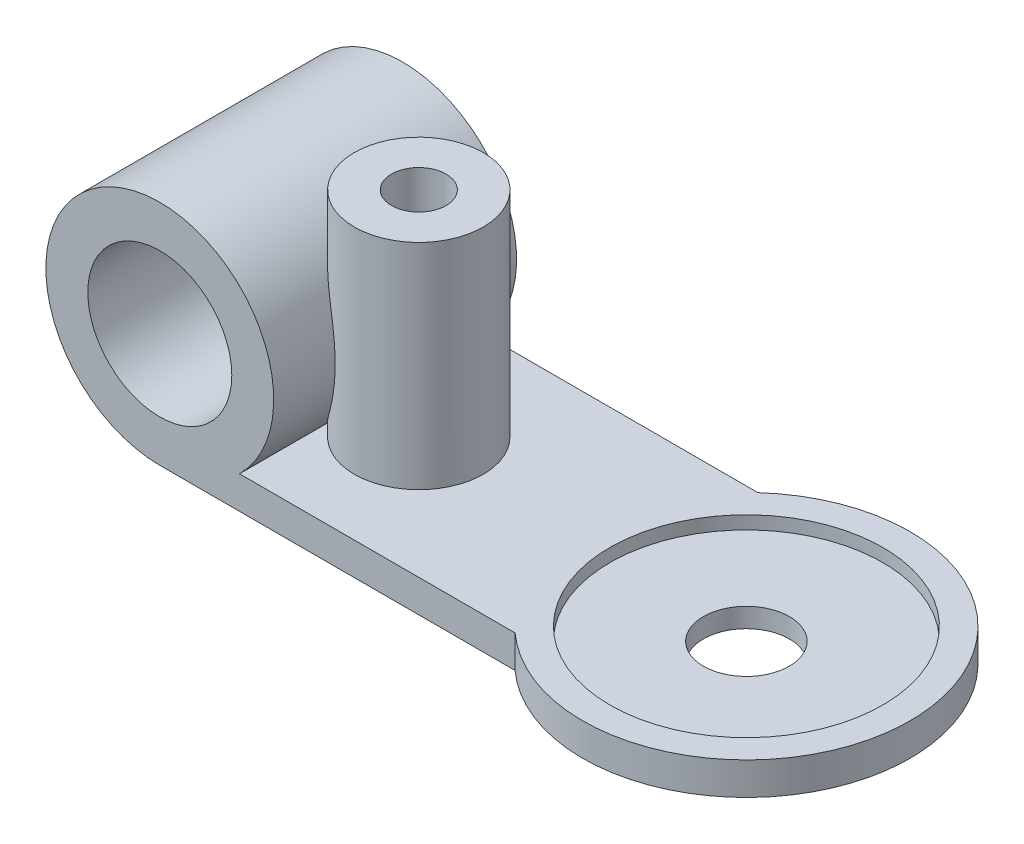
ISO-10303-21;
HEADER;
FILE_DESCRIPTION(('STEP AP214'),'2;1');
FILE_NAME('part.step','',(''),(''),'','','');
FILE_SCHEMA(('AUTOMOTIVE_DESIGN { 1 0 10303 214 1 1 1 1 }'));
ENDSEC;
DATA;
#1=APPLICATION_CONTEXT('core data for automotive mechanical design processes');
#2=APPLICATION_PROTOCOL_DEFINITION('international standard','automotive_design',2000,#1);
#3=PRODUCT_CONTEXT('',#1,'mechanical');
#4=PRODUCT('Part','Part','',(#3));
#5=PRODUCT_RELATED_PRODUCT_CATEGORY('part','',(#4));
#6=PRODUCT_DEFINITION_FORMATION('','',#4);
#7=PRODUCT_DEFINITION_CONTEXT('part definition',#1,'design');
#8=PRODUCT_DEFINITION('design','',#6,#7);
#9=PRODUCT_DEFINITION_SHAPE('','',#8);
#10=(LENGTH_UNIT() NAMED_UNIT(*) SI_UNIT(.MILLI.,.METRE.));
#11=(NAMED_UNIT(*) PLANE_ANGLE_UNIT() SI_UNIT($,.RADIAN.));
#12=(NAMED_UNIT(*) SI_UNIT($,.STERADIAN.) SOLID_ANGLE_UNIT());
#13=UNCERTAINTY_MEASURE_WITH_UNIT(LENGTH_MEASURE(1.E-05),#10,'distance_accuracy_value','');
#14=(GEOMETRIC_REPRESENTATION_CONTEXT(3) GLOBAL_UNCERTAINTY_ASSIGNED_CONTEXT((#13)) GLOBAL_UNIT_ASSIGNED_CONTEXT((#10,
#11,#12)) REPRESENTATION_CONTEXT('',''));
#15=CARTESIAN_POINT('',(0.,0.,0.));
#16=DIRECTION('',(0.,0.,1.));
#17=DIRECTION('',(1.,0.,0.));
#18=AXIS2_PLACEMENT_3D('',#15,#16,#17);
#19=CARTESIAN_POINT('',(0.,0.,28.25));
#20=DIRECTION('',(0.,0.,-1.));
#21=DIRECTION('',(-1.,0.,0.));
#22=AXIS2_PLACEMENT_3D('',#19,#20,#21);
#23=CYLINDRICAL_SURFACE('',#22,26.5);
#24=CARTESIAN_POINT('',(18.5395732151525,-18.935,-6.61943432400085));
#25=CARTESIAN_POINT('',(18.6184844088422,-18.857735922678,-6.7799048417251));
#26=CARTESIAN_POINT('',(18.6996500765237,-18.7772995053579,-6.93769789286287));
#27=CARTESIAN_POINT('',(18.8660127366865,-18.6101446090685,-7.24771071947177));
#28=CARTESIAN_POINT('',(18.9512093342821,-18.5234267450141,-7.39993103828863));
#29=CARTESIAN_POINT('',(19.2119367337667,-18.254144759126,-7.84758026850834));
#30=CARTESIAN_POINT('',(19.3928037608263,-18.0622597774062,-8.13439757428924));
#31=CARTESIAN_POINT('',(19.7627998857865,-17.6566247189803,-8.68095188456506));
#32=CARTESIAN_POINT('',(19.951837020215,-17.4430934524195,-8.94091496085011));
#33=CARTESIAN_POINT('',(20.3357805115592,-16.9939196843523,-9.43632416262915));
#34=CARTESIAN_POINT('',(20.5306880072531,-16.7582728736955,-9.67176549119735));
#35=CARTESIAN_POINT('',(20.9218465097154,-16.2672836439004,-10.1174184499874));
#36=CARTESIAN_POINT('',(21.1180906942836,-16.0120109229411,-10.3277131495032));
#37=CARTESIAN_POINT('',(21.5091176828609,-15.4827681042641,-10.7246923720679));
#38=CARTESIAN_POINT('',(21.7039005618658,-15.2087989734533,-10.9113781146592));
#39=CARTESIAN_POINT('',(22.0893971655171,-14.6432876309621,-11.2626874504629));
#40=CARTESIAN_POINT('',(22.2801010802677,-14.3517083671837,-11.4272619984179));
#41=CARTESIAN_POINT('',(22.654420937027,-13.7532508238555,-11.7353706091408));
#42=CARTESIAN_POINT('',(22.8380352807777,-13.4463691298775,-11.8788999476885));
#43=CARTESIAN_POINT('',(23.2748416317101,-12.6807752021044,-12.2055472513245));
#44=CARTESIAN_POINT('',(23.5230474379595,-12.2147374879152,-12.3782473299468));
#45=CARTESIAN_POINT('',(23.995092560242,-11.259213422958,-12.6886290410036));
#46=CARTESIAN_POINT('',(24.2189226548008,-10.7697182982629,-12.8262974468949));
#47=CARTESIAN_POINT('',(24.6387874594659,-9.77107435442968,-13.0717923879554));
#48=CARTESIAN_POINT('',(24.8347902467419,-9.26190380211747,-13.1795847828578));
#49=CARTESIAN_POINT('',(25.1961346386176,-8.22828073390988,-13.3697078714785));
#50=CARTESIAN_POINT('',(25.3614787423587,-7.70382946765761,-13.4520406409029));
#51=CARTESIAN_POINT('',(25.6629820174316,-6.63160021158971,-13.5967189298012));
#52=CARTESIAN_POINT('',(25.7984409213751,-6.08356320786244,-13.6585990242412));
#53=CARTESIAN_POINT('',(26.0343347911313,-4.97823420208279,-13.7632654845402));
#54=CARTESIAN_POINT('',(26.1347693571546,-4.42094209446301,-13.8060516324506));
#55=CARTESIAN_POINT('',(26.299813137327,-3.3001043780399,-13.8750090033395));
#56=CARTESIAN_POINT('',(26.364424374345,-2.73655912417212,-13.9011811644874));
#57=CARTESIAN_POINT('',(26.4573738854935,-1.60597799225613,-13.9384992548715));
#58=CARTESIAN_POINT('',(26.4857095319384,-1.03894186432941,-13.9496440955807));
#59=CARTESIAN_POINT('',(26.5078093563906,0.203223899776678,-13.958373278112));
#60=CARTESIAN_POINT('',(26.4940253741838,0.878523476463438,-13.9529958055844));
#61=CARTESIAN_POINT('',(26.4149873898834,2.22572657129171,-13.9215445875143));
#62=CARTESIAN_POINT('',(26.3497242849237,2.89762946766144,-13.8954671816726));
#63=CARTESIAN_POINT('',(26.1683420326795,4.23347916225571,-13.8203261304445));
#64=CARTESIAN_POINT('',(26.0522068975488,4.89742339181677,-13.7712552584307));
#65=CARTESIAN_POINT('',(25.7703712870232,6.21204961253387,-13.6460822837533));
#66=CARTESIAN_POINT('',(25.6046827022424,6.86273474531713,-13.5699866650013));
#67=CARTESIAN_POINT('',(25.262447074235,8.0218746786048,-13.4027671249236));
#68=CARTESIAN_POINT('',(25.0941300790476,8.53359687122828,-13.3173559684344));
#69=CARTESIAN_POINT('',(24.7284105075764,9.54164723509498,-13.1212454428095));
#70=CARTESIAN_POINT('',(24.5310086692119,10.0379757965075,-13.0105467152123));
#71=CARTESIAN_POINT('',(24.1100286586746,11.0107649833004,-12.7596350040241));
#72=CARTESIAN_POINT('',(23.8864936926616,11.4872566844235,-12.6194704386688));
#73=CARTESIAN_POINT('',(23.4166101032741,12.4170603194669,-12.3046876663241));
#74=CARTESIAN_POINT('',(23.1702676713678,12.8703784926649,-12.1300787953499));
#75=CARTESIAN_POINT('',(22.7201162927651,13.6454080938926,-11.7874377729025));
#76=CARTESIAN_POINT('',(22.5200103798547,13.9729076291405,-11.627599760965));
#77=CARTESIAN_POINT('',(22.1122791244786,14.6095823538444,-11.2829172598419));
#78=CARTESIAN_POINT('',(21.9046547033673,14.91875977642,-11.0980758271531));
#79=CARTESIAN_POINT('',(21.4853799374227,15.5164976378468,-10.7016793988646));
#80=CARTESIAN_POINT('',(21.2737306534324,15.8050634165476,-10.4901313617245));
#81=CARTESIAN_POINT('',(20.8503990749426,16.3594775351247,-10.0390259487247));
#82=CARTESIAN_POINT('',(20.6387167800646,16.6253255919709,-9.79946822399256));
#83=CARTESIAN_POINT('',(20.2178949693312,17.1346697648565,-9.28936592768098));
#84=CARTESIAN_POINT('',(20.0087988039591,17.3779291701216,-9.01854823991235));
#85=CARTESIAN_POINT('',(19.6002929103845,17.8374063186488,-8.44809405366109));
#86=CARTESIAN_POINT('',(19.400883447161,18.053623322423,-8.14845676748823));
#87=CARTESIAN_POINT('',(19.0170580950584,18.4574950885302,-7.52184269120322));
#88=CARTESIAN_POINT('',(18.8326340184803,18.645165497671,-7.1948810313701));
#89=CARTESIAN_POINT('',(18.4837019091153,18.9911344401795,-6.51577437651944));
#90=CARTESIAN_POINT('',(18.3191902538005,19.149438318795,-6.16363398069237));
#91=CARTESIAN_POINT('',(18.0376597305686,19.4145403441414,-5.49225574508178));
#92=CARTESIAN_POINT('',(17.9172206804698,19.5255067012741,-5.17608538709026));
#93=CARTESIAN_POINT('',(17.6963788383975,19.7258821825139,-4.53021502732));
#94=CARTESIAN_POINT('',(17.5959739211067,19.8152935934832,-4.20051646515699));
#95=CARTESIAN_POINT('',(17.417219800826,19.9725973456294,-3.5302701569404));
#96=CARTESIAN_POINT('',(17.3388657505196,20.040494416595,-3.1897248136242));
#97=CARTESIAN_POINT('',(17.2057274011577,20.1549168140827,-2.5005306640576));
#98=CARTESIAN_POINT('',(17.1509422706179,20.2014428945526,-2.15188214413536));
#99=CARTESIAN_POINT('',(17.0692809992501,20.2704775114588,-1.47656616277678));
#100=CARTESIAN_POINT('',(17.0405775733746,20.2945622406503,-1.15027837915579));
#101=CARTESIAN_POINT('',(17.0046109522173,20.324708287713,-0.495707506228005));
#102=CARTESIAN_POINT('',(16.9973463674244,20.3307707736563,-0.167424547616068));
#103=CARTESIAN_POINT('',(17.0043737178213,20.3248934226869,0.488675475588926));
#104=CARTESIAN_POINT('',(17.0186609760707,20.3129574915899,0.816492625815231));
#105=CARTESIAN_POINT('',(17.0685499043436,20.2710548088127,1.46934356410609));
#106=CARTESIAN_POINT('',(17.1041517014378,20.2410879496377,1.79437733556529));
#107=CARTESIAN_POINT('',(17.1954676147747,20.1635666797027,2.43497322147078));
#108=CARTESIAN_POINT('',(17.250905995754,20.116253181148,2.75060388717044));
#109=CARTESIAN_POINT('',(17.3810615753753,20.0039016310697,3.37464478181476));
#110=CARTESIAN_POINT('',(17.455778418004,19.9388639068565,3.68305514398136));
#111=CARTESIAN_POINT('',(17.623259902405,19.7909872194472,4.2905247000085));
#112=CARTESIAN_POINT('',(17.7160226297786,19.708150144399,4.58958488188071));
#113=CARTESIAN_POINT('',(17.9180671504668,19.5246377445448,5.1764346452842));
#114=CARTESIAN_POINT('',(18.0273491112994,19.4239622388412,5.46422411248432));
#115=CARTESIAN_POINT('',(18.2619822444088,19.2035465194546,6.03007256263128));
#116=CARTESIAN_POINT('',(18.3875068258975,19.0835965861395,6.307977865608));
#117=CARTESIAN_POINT('',(18.6514674019235,18.8256949946733,6.84888685637652));
#118=CARTESIAN_POINT('',(18.7899033820195,18.687743356657,7.11189056083507));
#119=CARTESIAN_POINT('',(19.0773641378205,18.3941936286244,7.62175437585969));
#120=CARTESIAN_POINT('',(19.2263890452499,18.2385953190721,7.86861428552619));
#121=CARTESIAN_POINT('',(19.5325902047457,17.9102847120049,8.3452955298152));
#122=CARTESIAN_POINT('',(19.6897667445542,17.7375718101706,8.57511626227991));
#123=CARTESIAN_POINT('',(20.0189182945683,17.3654268977745,9.02977678325369));
#124=CARTESIAN_POINT('',(20.19122634964,17.1650334919792,9.25358796116088));
#125=CARTESIAN_POINT('',(20.5393387023733,16.7469270905165,9.68139018006853));
#126=CARTESIAN_POINT('',(20.7151430488546,16.5292138528804,9.88538094407724));
#127=CARTESIAN_POINT('',(21.0676179586593,16.077547448731,10.2738425420623));
#128=CARTESIAN_POINT('',(21.2442887692305,15.8435893618977,10.4583074188573));
#129=CARTESIAN_POINT('',(21.5960121400256,15.3607151174697,10.8082657515267));
#130=CARTESIAN_POINT('',(21.7710643635481,15.1117959249711,10.9737553382766));
#131=CARTESIAN_POINT('',(22.1919076197606,14.4901396022377,11.3539767546389));
#132=CARTESIAN_POINT('',(22.4357113665878,14.1102286968233,11.5592396255565));
#133=CARTESIAN_POINT('',(22.9101285890656,13.3261485945659,11.9359154748766));
#134=CARTESIAN_POINT('',(23.1407375070773,12.9219711133948,12.1073168066764));
#135=CARTESIAN_POINT('',(23.5849744833405,12.0921816751011,12.4201978268302));
#136=CARTESIAN_POINT('',(23.7985692568709,11.6665302414797,12.5616197224473));
#137=CARTESIAN_POINT('',(24.2051127274323,10.7978085192994,12.817856433309));
#138=CARTESIAN_POINT('',(24.3980609002107,10.3547377888251,12.9326705730235));
#139=CARTESIAN_POINT('',(24.8128167805679,9.32542017307616,13.1687758539188));
#140=CARTESIAN_POINT('',(25.0271327429532,8.73441655369342,13.282554824441));
#141=CARTESIAN_POINT('',(25.4143409445632,7.53388798058901,13.4787299773193));
#142=CARTESIAN_POINT('',(25.5872218802748,6.92435802384971,13.5611175996938));
#143=CARTESIAN_POINT('',(25.8893506697452,5.69160323638436,13.6999125515157));
#144=CARTESIAN_POINT('',(26.0185906062613,5.06837594254059,13.7563151675027));
#145=CARTESIAN_POINT('',(26.2320119109073,3.81275780187263,13.8471566939317));
#146=CARTESIAN_POINT('',(26.3161963916898,3.18036759116877,13.8815971216613));
#147=CARTESIAN_POINT('',(26.4394600933486,1.90301362267372,13.931434709786));
#148=CARTESIAN_POINT('',(26.4780015872223,1.25798925071345,13.9466049939158));
#149=CARTESIAN_POINT('',(26.5078476183657,-0.0333325794905674,13.958385281654));
#150=CARTESIAN_POINT('',(26.4991512356277,-0.679630062284439,13.9549949237742));
#151=CARTESIAN_POINT('',(26.4345707121777,-1.9701022355119,13.9293643129771));
#152=CARTESIAN_POINT('',(26.3786410059838,-2.61427427293047,13.9071058581307));
#153=CARTESIAN_POINT('',(26.2200062618439,-3.89589512483408,13.8419329699027));
#154=CARTESIAN_POINT('',(26.1173003946484,-4.53334381992249,13.7990181703239));
#155=CARTESIAN_POINT('',(25.9246558906367,-5.50281050187106,13.7147878599766));
#156=CARTESIAN_POINT('',(25.8510212900026,-5.83890599472581,13.6820233130015));
#157=CARTESIAN_POINT('',(25.6909407573669,-6.507192511288,13.6089512090355));
#158=CARTESIAN_POINT('',(25.6044961623733,-6.83938393857092,13.5686444391283));
#159=CARTESIAN_POINT('',(25.4190613617537,-7.49925538378982,13.4796815851508));
#160=CARTESIAN_POINT('',(25.3200663459398,-7.82693361829073,13.4310222972743));
#161=CARTESIAN_POINT('',(25.1099615835061,-8.47681696372066,13.3244604680227));
#162=CARTESIAN_POINT('',(24.998853508059,-8.79902282257208,13.2665592012026));
#163=CARTESIAN_POINT('',(24.7652382888835,-9.43652400491347,13.1406162953713));
#164=CARTESIAN_POINT('',(24.6427541117748,-9.75183172946336,13.0725949270249));
#165=CARTESIAN_POINT('',(24.3868426100582,-10.3752307809703,12.9252323993235));
#166=CARTESIAN_POINT('',(24.2534170263344,-10.6833232459554,12.845893039291));
#167=CARTESIAN_POINT('',(23.9764503516102,-11.2912050255229,12.6747440431043));
#168=CARTESIAN_POINT('',(23.8329145397696,-11.5909985612139,12.5829408921581));
#169=CARTESIAN_POINT('',(23.5366564982352,-12.1813328278583,12.3856159853349));
#170=CARTESIAN_POINT('',(23.3839357165304,-12.4718750062785,12.2800963887932));
#171=CARTESIAN_POINT('',(23.0346564364344,-13.1078001669069,12.0282571100051));
#172=CARTESIAN_POINT('',(22.8360478726092,-13.4505655717285,11.8781220143143));
#173=CARTESIAN_POINT('',(22.4294173458473,-14.1182149337593,11.5529941889334));
#174=CARTESIAN_POINT('',(22.22139704328,-14.4431020227268,11.378005832163));
#175=CARTESIAN_POINT('',(21.7998749792299,-15.071768991268,11.0016820407517));
#176=CARTESIAN_POINT('',(21.5863919094892,-15.3756103337218,10.8004287475765));
#177=CARTESIAN_POINT('',(21.1572777006362,-15.9609291730894,10.3695598770521));
#178=CARTESIAN_POINT('',(20.9416466215977,-16.2424072934759,10.13994509086));
#179=CARTESIAN_POINT('',(20.5313297351304,-16.7574882218179,9.67252569858841));
#180=CARTESIAN_POINT('',(20.3364438449534,-16.9931262380019,9.43714249801635));
#181=CARTESIAN_POINT('',(19.9525468045447,-17.442280433207,8.94186823962059));
#182=CARTESIAN_POINT('',(19.7635341172648,-17.6558024348246,8.68198366699395));
#183=CARTESIAN_POINT('',(19.3934250818023,-18.061596045778,8.13536847248127));
#184=CARTESIAN_POINT('',(19.2124288738738,-18.2536292764721,7.84839155608623));
#185=CARTESIAN_POINT('',(18.9515131373651,-18.5231165712909,7.40046947406409));
#186=CARTESIAN_POINT('',(18.8662519380489,-18.6099026709269,7.24814713766491));
#187=CARTESIAN_POINT('',(18.6997653932826,-18.7771852320824,6.93792209508578));
#188=CARTESIAN_POINT('',(18.618540445994,-18.8576810735377,6.78001884098767));
#189=CARTESIAN_POINT('',(18.5395732151524,-18.9350000000003,6.6194343240013));
#190=B_SPLINE_CURVE_WITH_KNOTS('',3,(#24,#25,#26,#27,#28,#29,#30,#31,#32,#33,#34,#35,#36,#37,
#38,#39,#40,#41,#42,#43,#44,#45,#46,#47,#48,#49,#50,#51,#52,#53,#54,#55,#56,#57,#58,#59,#60,#61,
#62,#63,#64,#65,#66,#67,#68,#69,#70,#71,#72,#73,#74,#75,#76,#77,#78,#79,#80,#81,#82,#83,#84,#85,
#86,#87,#88,#89,#90,#91,#92,#93,#94,#95,#96,#97,#98,#99,#100,#101,#102,#103,#104,#105,#106,#107,
#108,#109,#110,#111,#112,#113,#114,#115,#116,#117,#118,#119,#120,#121,#122,#123,#124,#125,#126,
#127,#128,#129,#130,#131,#132,#133,#134,#135,#136,#137,#138,#139,#140,#141,#142,#143,#144,#145,
#146,#147,#148,#149,#150,#151,#152,#153,#154,#155,#156,#157,#158,#159,#160,#161,#162,#163,#164,
#165,#166,#167,#168,#169,#170,#171,#172,#173,#174,#175,#176,#177,#178,#179,#180,#181,#182,#183,
#184,#185,#186,#187,#188,#189),.UNSPECIFIED.,.F.,.F.,(4,2,2,2,2,2,2,2,2,2,2,2,2,2,2,2,2,2,2,2,2,
2,2,2,2,2,2,2,2,2,2,2,2,2,2,2,2,2,2,2,2,2,2,2,2,2,2,2,2,2,2,2,2,2,2,2,2,2,2,2,2,2,2,2,2,2,2,2,2,
2,2,2,2,2,2,2,2,2,2,2,2,2,4),(0.,0.584281773984408,1.16850642749218,2.33550248375017,
3.49169740481286,4.64811807672346,5.80060642788943,6.95303522187347,8.10797946246583,
9.26318256886644,10.9273351934287,12.5921152055789,14.2587898440107,15.9253285637394,
17.6275306995802,19.32975226477,21.0318776992502,22.7341264231758,24.7581743998584,
26.7825803618394,28.8076230025236,30.8321801127742,32.4670100560912,34.1017985288416,
35.7339214272595,37.3656025505078,38.6117504631279,39.8577461801456,41.1034179179208,
42.3491051727072,43.6066434804189,44.8642161686335,46.1210970595373,47.3777489500863,
48.4445332758727,49.5112043718016,50.5776408040179,51.6440396105031,52.6281550988669,
53.6122068025575,54.5960449890501,55.5798890409347,56.5505571703639,57.5212073758405,
58.4917546659359,59.462311798804,60.4442502456279,61.4261875941773,62.4081371600057,
63.3901214110198,64.4280160386437,65.4659251688362,66.5041500490447,67.5425862516873,
69.0280415942568,70.5140069698374,72.0028113707496,73.4916535659881,75.4056313990561,
77.3201307742282,79.2349772868027,81.1496914952755,83.0867456847497,85.0238376005437,
86.9628003456221,88.9017974660378,89.938382844079,90.974860107466,92.0117358282868,
93.048468677612,94.0831522220019,95.1176714564295,96.1516544541728,97.1854748720284,
98.4552422895846,99.7247865682927,100.990451557015,102.256081247392,103.412367410513,
104.568348374291,105.736093695004,106.320732890495,106.905429644468),.UNSPECIFIED.);
#191=CARTESIAN_POINT('',(18.5395732151525,-18.935,-6.61943432400081));
#192=VERTEX_POINT('',#191);
#193=CARTESIAN_POINT('',(18.5395732151525,-18.935,6.61943432400081));
#194=VERTEX_POINT('',#193);
#195=EDGE_CURVE('E53',#192,#194,#190,.T.);
#196=ORIENTED_EDGE('',*,*,#195,.F.);
#197=DIRECTION('',(0.,0.,1.));
#198=VECTOR('',#197,1.);
#199=CARTESIAN_POINT('',(18.5395732151525,-18.935,-28.25));
#200=LINE('',#199,#198);
#201=CARTESIAN_POINT('',(18.5395732151525,-18.935,-28.25));
#202=VERTEX_POINT('',#201);
#203=EDGE_CURVE('E88',#202,#192,#200,.T.);
#204=ORIENTED_EDGE('',*,*,#203,.F.);
#205=CARTESIAN_POINT('',(0.,0.,-28.25));
#206=DIRECTION('',(0.,0.,1.));
#207=DIRECTION('',(1.,0.,0.));
#208=AXIS2_PLACEMENT_3D('',#205,#206,#207);
#209=CIRCLE('',#208,26.5);
#210=CARTESIAN_POINT('',(0.,-26.5,-28.25));
#211=VERTEX_POINT('',#210);
#212=EDGE_CURVE('E111',#202,#211,#209,.T.);
#213=ORIENTED_EDGE('',*,*,#212,.T.);
#214=DIRECTION('',(0.,0.,1.));
#215=VECTOR('',#214,1.);
#216=CARTESIAN_POINT('',(0.,-26.5,-28.25));
#217=LINE('',#216,#215);
#218=CARTESIAN_POINT('',(0.,-26.5,28.25));
#219=VERTEX_POINT('',#218);
#220=EDGE_CURVE('E101',#211,#219,#217,.T.);
#221=ORIENTED_EDGE('',*,*,#220,.T.);
#222=CARTESIAN_POINT('',(0.,0.,28.25));
#223=DIRECTION('',(0.,0.,1.));
#224=DIRECTION('',(1.,0.,0.));
#225=AXIS2_PLACEMENT_3D('',#222,#223,#224);
#226=CIRCLE('',#225,26.5);
#227=CARTESIAN_POINT('',(18.5395732151525,-18.935,28.25));
#228=VERTEX_POINT('',#227);
#229=EDGE_CURVE('E113',#228,#219,#226,.T.);
#230=ORIENTED_EDGE('',*,*,#229,.F.);
#231=EDGE_CURVE('E58',#194,#228,#200,.T.);
#232=ORIENTED_EDGE('',*,*,#231,.F.);
#233=EDGE_LOOP('',(#196,#204,#213,#221,#230,#232));
#234=FACE_BOUND('',#233,.T.);
#235=ADVANCED_FACE('F39',(#234),#23,.T.);
#236=CARTESIAN_POINT('',(0.,0.,28.25));
#237=DIRECTION('',(0.,0.,1.));
#238=DIRECTION('',(1.,0.,0.));
#239=AXIS2_PLACEMENT_3D('',#236,#237,#238);
#240=PLANE('',#239);
#241=DIRECTION('',(0.,1.,0.));
#242=VECTOR('',#241,1.);
#243=CARTESIAN_POINT('',(82.6354249008515,-26.5,28.25));
#244=LINE('',#243,#242);
#245=CARTESIAN_POINT('',(82.6354249008515,-18.935,28.25));
#246=VERTEX_POINT('',#245);
#247=CARTESIAN_POINT('',(82.6354249008515,-26.5,28.25));
#248=VERTEX_POINT('',#247);
#249=EDGE_CURVE('E185',#246,#248,#244,.F.);
#250=ORIENTED_EDGE('',*,*,#249,.F.);
#251=DIRECTION('',(-1.,0.,0.));
#252=VECTOR('',#251,1.);
#253=CARTESIAN_POINT('',(108.2,-18.935,28.25));
#254=LINE('',#253,#252);
#255=EDGE_CURVE('E106',#246,#228,#254,.T.);
#256=ORIENTED_EDGE('',*,*,#255,.T.);
#257=ORIENTED_EDGE('',*,*,#229,.T.);
#258=DIRECTION('',(1.,0.,0.));
#259=VECTOR('',#258,1.);
#260=CARTESIAN_POINT('',(0.,-26.5,28.25));
#261=LINE('',#260,#259);
#262=EDGE_CURVE('E179',#219,#248,#261,.T.);
#263=ORIENTED_EDGE('',*,*,#262,.T.);
#264=EDGE_LOOP('',(#250,#256,#257,#263));
#265=FACE_BOUND('',#264,.T.);
#266=CARTESIAN_POINT('',(0.,0.,28.25));
#267=DIRECTION('',(0.,0.,1.));
#268=DIRECTION('',(1.,0.,0.));
#269=AXIS2_PLACEMENT_3D('',#266,#267,#268);
#270=CIRCLE('',#269,16.75);
#271=CARTESIAN_POINT('',(16.75,0.,28.25));
#272=VERTEX_POINT('',#271);
#273=EDGE_CURVE('E103',#272,#272,#270,.T.);
#274=ORIENTED_EDGE('',*,*,#273,.F.);
#275=EDGE_LOOP('',(#274));
#276=FACE_BOUND('',#275,.T.);
#277=ADVANCED_FACE('F136',(#265,#276),#240,.T.);
#278=CARTESIAN_POINT('',(0.,0.,-28.25));
#279=DIRECTION('',(0.,0.,1.));
#280=DIRECTION('',(1.,0.,0.));
#281=AXIS2_PLACEMENT_3D('',#278,#279,#280);
#282=PLANE('',#281);
#283=DIRECTION('',(-1.,0.,0.));
#284=VECTOR('',#283,1.);
#285=CARTESIAN_POINT('',(108.2,-18.935,-28.25));
#286=LINE('',#285,#284);
#287=CARTESIAN_POINT('',(82.6354249008515,-18.935,-28.25));
#288=VERTEX_POINT('',#287);
#289=EDGE_CURVE('E97',#288,#202,#286,.T.);
#290=ORIENTED_EDGE('',*,*,#289,.F.);
#291=DIRECTION('',(0.,1.,0.));
#292=VECTOR('',#291,1.);
#293=CARTESIAN_POINT('',(82.6354249008515,-26.5,-28.25));
#294=LINE('',#293,#292);
#295=CARTESIAN_POINT('',(82.6354249008515,-26.5,-28.25));
#296=VERTEX_POINT('',#295);
#297=EDGE_CURVE('E183',#288,#296,#294,.F.);
#298=ORIENTED_EDGE('',*,*,#297,.T.);
#299=DIRECTION('',(1.,0.,0.));
#300=VECTOR('',#299,1.);
#301=CARTESIAN_POINT('',(0.,-26.5,-28.25));
#302=LINE('',#301,#300);
#303=EDGE_CURVE('E172',#211,#296,#302,.T.);
#304=ORIENTED_EDGE('',*,*,#303,.F.);
#305=ORIENTED_EDGE('',*,*,#212,.F.);
#306=EDGE_LOOP('',(#290,#298,#304,#305));
#307=FACE_BOUND('',#306,.T.);
#308=CARTESIAN_POINT('',(0.,0.,-28.25));
#309=DIRECTION('',(0.,0.,1.));
#310=DIRECTION('',(1.,0.,0.));
#311=AXIS2_PLACEMENT_3D('',#308,#309,#310);
#312=CIRCLE('',#311,16.75);
#313=CARTESIAN_POINT('',(16.75,0.,-28.25));
#314=VERTEX_POINT('',#313);
#315=EDGE_CURVE('E96',#314,#314,#312,.T.);
#316=ORIENTED_EDGE('',*,*,#315,.T.);
#317=EDGE_LOOP('',(#316));
#318=FACE_BOUND('',#317,.T.);
#319=ADVANCED_FACE('F143',(#307,#318),#282,.F.);
#320=CARTESIAN_POINT('',(0.,0.,28.25));
#321=DIRECTION('',(0.,0.,-1.));
#322=DIRECTION('',(-1.,0.,0.));
#323=AXIS2_PLACEMENT_3D('',#320,#321,#322);
#324=CYLINDRICAL_SURFACE('',#323,16.75);
#325=ORIENTED_EDGE('',*,*,#273,.T.);
#326=EDGE_LOOP('',(#325));
#327=FACE_BOUND('',#326,.T.);
#328=ORIENTED_EDGE('',*,*,#315,.F.);
#329=EDGE_LOOP('',(#328));
#330=FACE_BOUND('',#329,.T.);
#331=ADVANCED_FACE('F140',(#327,#330),#324,.F.);
#332=CARTESIAN_POINT('',(108.2,-18.935,-28.25));
#333=DIRECTION('',(0.,1.,0.));
#334=DIRECTION('',(0.,0.,1.));
#335=AXIS2_PLACEMENT_3D('',#332,#333,#334);
#336=PLANE('',#335);
#337=CARTESIAN_POINT('',(108.2,-18.935,0.));
#338=DIRECTION('',(0.,1.,0.));
#339=DIRECTION('',(0.,0.,1.));
#340=AXIS2_PLACEMENT_3D('',#337,#338,#339);
#341=CIRCLE('',#340,31.75);
#342=CARTESIAN_POINT('',(108.2,-18.935,31.75));
#343=VERTEX_POINT('',#342);
#344=EDGE_CURVE('E192',#343,#343,#341,.T.);
#345=ORIENTED_EDGE('',*,*,#344,.F.);
#346=EDGE_LOOP('',(#345));
#347=FACE_BOUND('',#346,.T.);
#348=ORIENTED_EDGE('',*,*,#203,.T.);
#349=CARTESIAN_POINT('',(32.,-18.935,0.));
#350=DIRECTION('',(0.,1.,0.));
#351=DIRECTION('',(0.,0.,1.));
#352=AXIS2_PLACEMENT_3D('',#349,#350,#351);
#353=CIRCLE('',#352,15.);
#354=EDGE_CURVE('E11',#192,#194,#353,.F.);
#355=ORIENTED_EDGE('',*,*,#354,.T.);
#356=ORIENTED_EDGE('',*,*,#231,.T.);
#357=ORIENTED_EDGE('',*,*,#255,.F.);
#358=CARTESIAN_POINT('',(108.2,-18.935,0.));
#359=DIRECTION('',(0.,-1.,0.));
#360=DIRECTION('',(0.,0.,-1.));
#361=AXIS2_PLACEMENT_3D('',#358,#359,#360);
#362=CIRCLE('',#361,38.1);
#363=EDGE_CURVE('E187',#246,#288,#362,.F.);
#364=ORIENTED_EDGE('',*,*,#363,.T.);
#365=ORIENTED_EDGE('',*,*,#289,.T.);
#366=EDGE_LOOP('',(#348,#355,#356,#357,#364,#365));
#367=FACE_BOUND('',#366,.T.);
#368=ADVANCED_FACE('F91',(#347,#367),#336,.T.);
#369=CARTESIAN_POINT('',(0.,-26.5,-28.25));
#370=DIRECTION('',(0.,-1.,0.));
#371=DIRECTION('',(0.,0.,-1.));
#372=AXIS2_PLACEMENT_3D('',#369,#370,#371);
#373=PLANE('',#372);
#374=CARTESIAN_POINT('',(108.2,-26.5,0.));
#375=DIRECTION('',(0.,1.,0.));
#376=DIRECTION('',(0.,0.,1.));
#377=AXIS2_PLACEMENT_3D('',#374,#375,#376);
#378=CIRCLE('',#377,9.99999999999999);
#379=CARTESIAN_POINT('',(108.2,-26.5,9.99999999999999));
#380=VERTEX_POINT('',#379);
#381=EDGE_CURVE('E167',#380,#380,#378,.T.);
#382=ORIENTED_EDGE('',*,*,#381,.T.);
#383=EDGE_LOOP('',(#382));
#384=FACE_BOUND('',#383,.T.);
#385=ORIENTED_EDGE('',*,*,#303,.T.);
#386=CARTESIAN_POINT('',(108.2,-26.5,0.));
#387=DIRECTION('',(0.,1.,0.));
#388=DIRECTION('',(0.,0.,1.));
#389=AXIS2_PLACEMENT_3D('',#386,#387,#388);
#390=CIRCLE('',#389,38.1);
#391=EDGE_CURVE('E174',#248,#296,#390,.T.);
#392=ORIENTED_EDGE('',*,*,#391,.F.);
#393=ORIENTED_EDGE('',*,*,#262,.F.);
#394=ORIENTED_EDGE('',*,*,#220,.F.);
#395=EDGE_LOOP('',(#385,#392,#393,#394));
#396=FACE_BOUND('',#395,.T.);
#397=ADVANCED_FACE('F137',(#384,#396),#373,.T.);
#398=CARTESIAN_POINT('',(108.2,-26.5,0.));
#399=DIRECTION('',(0.,1.,0.));
#400=DIRECTION('',(0.,0.,1.));
#401=AXIS2_PLACEMENT_3D('',#398,#399,#400);
#402=CYLINDRICAL_SURFACE('',#401,38.1);
#403=ORIENTED_EDGE('',*,*,#363,.F.);
#404=ORIENTED_EDGE('',*,*,#249,.T.);
#405=ORIENTED_EDGE('',*,*,#391,.T.);
#406=ORIENTED_EDGE('',*,*,#297,.F.);
#407=EDGE_LOOP('',(#403,#404,#405,#406));
#408=FACE_BOUND('',#407,.T.);
#409=ADVANCED_FACE('F158',(#408),#402,.T.);
#410=CARTESIAN_POINT('',(108.2,-21.985,0.));
#411=DIRECTION('',(0.,1.,0.));
#412=DIRECTION('',(0.,0.,1.));
#413=AXIS2_PLACEMENT_3D('',#410,#411,#412);
#414=CYLINDRICAL_SURFACE('',#413,31.75);
#415=CARTESIAN_POINT('',(108.2,-21.985,0.));
#416=DIRECTION('',(0.,1.,0.));
#417=DIRECTION('',(0.,0.,1.));
#418=AXIS2_PLACEMENT_3D('',#415,#416,#417);
#419=CIRCLE('',#418,31.75);
#420=CARTESIAN_POINT('',(108.2,-21.985,31.75));
#421=VERTEX_POINT('',#420);
#422=EDGE_CURVE('E188',#421,#421,#419,.T.);
#423=ORIENTED_EDGE('',*,*,#422,.F.);
#424=EDGE_LOOP('',(#423));
#425=FACE_BOUND('',#424,.T.);
#426=ORIENTED_EDGE('',*,*,#344,.T.);
#427=EDGE_LOOP('',(#426));
#428=FACE_BOUND('',#427,.T.);
#429=ADVANCED_FACE('F164',(#425,#428),#414,.F.);
#430=CARTESIAN_POINT('',(108.2,-21.985,0.));
#431=DIRECTION('',(0.,1.,0.));
#432=DIRECTION('',(0.,0.,1.));
#433=AXIS2_PLACEMENT_3D('',#430,#431,#432);
#434=PLANE('',#433);
#435=CARTESIAN_POINT('',(108.2,-21.985,0.));
#436=DIRECTION('',(0.,1.,0.));
#437=DIRECTION('',(0.,0.,1.));
#438=AXIS2_PLACEMENT_3D('',#435,#436,#437);
#439=CIRCLE('',#438,9.99999999999999);
#440=CARTESIAN_POINT('',(108.2,-21.985,9.99999999999999));
#441=VERTEX_POINT('',#440);
#442=EDGE_CURVE('E95',#441,#441,#439,.T.);
#443=ORIENTED_EDGE('',*,*,#442,.F.);
#444=EDGE_LOOP('',(#443));
#445=FACE_BOUND('',#444,.T.);
#446=ORIENTED_EDGE('',*,*,#422,.T.);
#447=EDGE_LOOP('',(#446));
#448=FACE_BOUND('',#447,.T.);
#449=ADVANCED_FACE('F213',(#445,#448),#434,.T.);
#450=CARTESIAN_POINT('',(108.2,-26.5,0.));
#451=DIRECTION('',(0.,1.,0.));
#452=DIRECTION('',(0.,0.,1.));
#453=AXIS2_PLACEMENT_3D('',#450,#451,#452);
#454=CYLINDRICAL_SURFACE('',#453,9.99999999999999);
#455=ORIENTED_EDGE('',*,*,#381,.F.);
#456=EDGE_LOOP('',(#455));
#457=FACE_BOUND('',#456,.T.);
#458=ORIENTED_EDGE('',*,*,#442,.T.);
#459=EDGE_LOOP('',(#458));
#460=FACE_BOUND('',#459,.T.);
#461=ADVANCED_FACE('F215',(#457,#460),#454,.F.);
#462=CARTESIAN_POINT('',(32.,30.88,0.));
#463=DIRECTION('',(0.,-1.,0.));
#464=DIRECTION('',(0.,0.,-1.));
#465=AXIS2_PLACEMENT_3D('',#462,#463,#464);
#466=CYLINDRICAL_SURFACE('',#465,15.);
#467=CARTESIAN_POINT('',(32.,30.88,0.));
#468=DIRECTION('',(0.,1.,0.));
#469=DIRECTION('',(0.,0.,1.));
#470=AXIS2_PLACEMENT_3D('',#467,#468,#469);
#471=CIRCLE('',#470,15.);
#472=CARTESIAN_POINT('',(32.,30.88,15.));
#473=VERTEX_POINT('',#472);
#474=EDGE_CURVE('E324',#473,#473,#471,.T.);
#475=ORIENTED_EDGE('',*,*,#474,.F.);
#476=EDGE_LOOP('',(#475));
#477=FACE_BOUND('',#476,.T.);
#478=ORIENTED_EDGE('',*,*,#354,.F.);
#479=ORIENTED_EDGE('',*,*,#195,.T.);
#480=EDGE_LOOP('',(#478,#479));
#481=FACE_BOUND('',#480,.T.);
#482=ADVANCED_FACE('F81',(#477,#481),#466,.T.);
#483=CARTESIAN_POINT('',(32.,30.88,0.));
#484=DIRECTION('',(0.,-1.,0.));
#485=DIRECTION('',(0.,0.,-1.));
#486=AXIS2_PLACEMENT_3D('',#483,#484,#485);
#487=CYLINDRICAL_SURFACE('',#486,6.35);
#488=CARTESIAN_POINT('',(32.,30.88,0.));
#489=DIRECTION('',(0.,1.,0.));
#490=DIRECTION('',(0.,0.,1.));
#491=AXIS2_PLACEMENT_3D('',#488,#489,#490);
#492=CIRCLE('',#491,6.35);
#493=CARTESIAN_POINT('',(32.,30.88,6.35));
#494=VERTEX_POINT('',#493);
#495=EDGE_CURVE('E322',#494,#494,#492,.T.);
#496=ORIENTED_EDGE('',*,*,#495,.T.);
#497=EDGE_LOOP('',(#496));
#498=FACE_BOUND('',#497,.T.);
#499=CARTESIAN_POINT('',(32.,-18.935,0.));
#500=DIRECTION('',(0.,1.,0.));
#501=DIRECTION('',(0.,0.,1.));
#502=AXIS2_PLACEMENT_3D('',#499,#500,#501);
#503=CIRCLE('',#502,6.35);
#504=CARTESIAN_POINT('',(32.,-18.935,6.35));
#505=VERTEX_POINT('',#504);
#506=EDGE_CURVE('E48',#505,#505,#503,.F.);
#507=ORIENTED_EDGE('',*,*,#506,.T.);
#508=EDGE_LOOP('',(#507));
#509=FACE_BOUND('',#508,.T.);
#510=CARTESIAN_POINT('',(26.5,0.,3.17372021451168));
#511=CARTESIAN_POINT('',(26.4999988285425,-0.339517756293321,3.17372690907424));
#512=CARTESIAN_POINT('',(26.4934655142194,-0.679074884099817,3.16247305464786));
#513=CARTESIAN_POINT('',(26.4674302742264,-1.35648824574887,3.11671306045008));
#514=CARTESIAN_POINT('',(26.4479168712434,-1.69434270742518,3.08218634188061));
#515=CARTESIAN_POINT('',(26.4092359838675,-2.19789028028274,3.01106996992672));
#516=CARTESIAN_POINT('',(26.3947570539096,-2.36534586792382,2.98411132056772));
#517=CARTESIAN_POINT('',(26.3627600904988,-2.6986826435735,2.92322134651475));
#518=CARTESIAN_POINT('',(26.34524253291,-2.86456407381912,2.88929111345166));
#519=CARTESIAN_POINT('',(26.3073259760688,-3.1940685637521,2.81384824664715));
#520=CARTESIAN_POINT('',(26.2869302871047,-3.35769398412638,2.77234430796238));
#521=CARTESIAN_POINT('',(26.2434444095756,-3.68217350294414,2.68088367234781));
#522=CARTESIAN_POINT('',(26.2203549882,-3.843028375549,2.63092938030886));
#523=CARTESIAN_POINT('',(26.1732918947375,-4.1510862679381,2.52490047110333));
#524=CARTESIAN_POINT('',(26.149465411812,-4.29851120123686,2.46940917755762));
#525=CARTESIAN_POINT('',(26.1000220455063,-4.58918031235027,2.34883272080964));
#526=CARTESIAN_POINT('',(26.0744045393072,-4.73242301102074,2.28374421141263));
#527=CARTESIAN_POINT('',(26.0220454072952,-5.01231422421,2.14293583652089));
#528=CARTESIAN_POINT('',(25.9953115063817,-5.14899734408152,2.06728256412216));
#529=CARTESIAN_POINT('',(25.9413397942987,-5.41434738187654,1.90331161378136));
#530=CARTESIAN_POINT('',(25.9141026469077,-5.54302400042082,1.81500970697204));
#531=CARTESIAN_POINT('',(25.8652982486892,-5.76600732594631,1.64147854559073));
#532=CARTESIAN_POINT('',(25.8436247049152,-5.86223687384308,1.55877261620165));
#533=CARTESIAN_POINT('',(25.8015866173395,-6.04457409583967,1.38217905847414));
#534=CARTESIAN_POINT('',(25.7812236750288,-6.13066948906706,1.28827813538052));
#535=CARTESIAN_POINT('',(25.7429237919341,-6.28956515735505,1.08724395834866));
#536=CARTESIAN_POINT('',(25.7250193473629,-6.36219111195997,0.979963739999889));
#537=CARTESIAN_POINT('',(25.6938386952022,-6.4869737390954,0.753491718582087));
#538=CARTESIAN_POINT('',(25.6805485809368,-6.53919197726182,0.634337124569223));
#539=CARTESIAN_POINT('',(25.663496950206,-6.60573557506923,0.423065465955846));
#540=CARTESIAN_POINT('',(25.6580884294182,-6.62666420758692,0.333161256217023));
#541=CARTESIAN_POINT('',(25.6511432556397,-6.653499340833,0.150987082361484));
#542=CARTESIAN_POINT('',(25.6496039323664,-6.65941620179076,0.0587187942361497));
#543=CARTESIAN_POINT('',(25.6505718073425,-6.65568684220006,-0.125530213061497));
#544=CARTESIAN_POINT('',(25.6530815196209,-6.64603095259876,-0.217510718016879));
#545=CARTESIAN_POINT('',(25.6618680032936,-6.61202152912805,-0.39852047543023));
#546=CARTESIAN_POINT('',(25.668147491615,-6.58765739476325,-0.487547550431887));
#547=CARTESIAN_POINT('',(25.6859386792372,-6.51798623668554,-0.683514961090938));
#548=CARTESIAN_POINT('',(25.6983926325245,-6.46885424956584,-0.789000636691997));
#549=CARTESIAN_POINT('',(25.726877208921,-6.35462506643367,-0.99037050151776));
#550=CARTESIAN_POINT('',(25.7429145427475,-6.28949789270152,-1.08623618044945));
#551=CARTESIAN_POINT('',(25.7861620649297,-6.11032565192099,-1.31552051794956));
#552=CARTESIAN_POINT('',(25.8148417703214,-5.9884669050218,-1.44250098118182));
#553=CARTESIAN_POINT('',(25.8740570954835,-5.72723771073342,-1.6762790708159));
#554=CARTESIAN_POINT('',(25.9045970788204,-5.58782520229428,-1.78302662378166));
#555=CARTESIAN_POINT('',(25.9626236001406,-5.31133106745674,-1.97007491811176));
#556=CARTESIAN_POINT('',(25.990125232264,-5.17528057268981,-2.05192326480058));
#557=CARTESIAN_POINT('',(26.0441020302325,-4.8964220267064,-2.20369453321098));
#558=CARTESIAN_POINT('',(26.0705763422194,-4.75360856442356,-2.27360769236756));
#559=CARTESIAN_POINT('',(26.1219137125603,-4.46289738743772,-2.40321910434022));
#560=CARTESIAN_POINT('',(26.1467740578765,-4.31499172036654,-2.46290042050602));
#561=CARTESIAN_POINT('',(26.1944407710022,-4.0155082806989,-2.57324178662418));
#562=CARTESIAN_POINT('',(26.2172464008178,-3.86392921333349,-2.6238986015728));
#563=CARTESIAN_POINT('',(26.2792837158716,-3.42525053665605,-2.75776328131734));
#564=CARTESIAN_POINT('',(26.3155960953603,-3.13469382874726,-2.83107180013438));
#565=CARTESIAN_POINT('',(26.378907615078,-2.54767179316538,-2.95475169318408));
#566=CARTESIAN_POINT('',(26.405899011929,-2.25120176823323,-3.00510400768489));
#567=CARTESIAN_POINT('',(26.4500119219178,-1.65426614579011,-3.08581372890835));
#568=CARTESIAN_POINT('',(26.4671141612254,-1.35379390562731,-3.1161321060655));
#569=CARTESIAN_POINT('',(26.4910641688353,-0.751282802273425,-3.15827417969859));
#570=CARTESIAN_POINT('',(26.4979153265971,-0.449244490055353,-3.17010398936772));
#571=CARTESIAN_POINT('',(26.5013872696532,0.176518727683918,-3.17612788387412));
#572=CARTESIAN_POINT('',(26.4972476556087,0.500261740170732,-3.16901104952838));
#573=CARTESIAN_POINT('',(26.4771662396253,1.14639320397584,-3.13388122959042));
#574=CARTESIAN_POINT('',(26.4612190882291,1.46878097469603,-3.10585877256954));
#575=CARTESIAN_POINT('',(26.4178362703908,2.10969704155578,-3.02721469103482));
#576=CARTESIAN_POINT('',(26.3904158686038,2.42822988925318,-2.97662308788204));
#577=CARTESIAN_POINT('',(26.3412010375906,2.90108438865987,-2.88127103961817));
#578=CARTESIAN_POINT('',(26.3234553039988,3.05783181314951,-2.84625643248418));
#579=CARTESIAN_POINT('',(26.2854110969894,3.36923408148673,-2.7690864178344));
#580=CARTESIAN_POINT('',(26.2651131222115,3.52388932757057,-2.72693240461103));
#581=CARTESIAN_POINT('',(26.2218099526032,3.83293826457208,-2.63395002301703));
#582=CARTESIAN_POINT('',(26.1987667922903,3.98728856706203,-2.58299420360261));
#583=CARTESIAN_POINT('',(26.1505348898785,4.29224121454362,-2.47182811921167));
#584=CARTESIAN_POINT('',(26.1253469797786,4.44284498387163,-2.41162143563727));
#585=CARTESIAN_POINT('',(26.0733425750887,4.73848439650728,-2.28082694475271));
#586=CARTESIAN_POINT('',(26.0465330929576,4.88354012886258,-2.21028218957099));
#587=CARTESIAN_POINT('',(25.9918344829332,5.16674842983618,-2.0569592761852));
#588=CARTESIAN_POINT('',(25.963946390564,5.30490734146706,-1.97419264653667));
#589=CARTESIAN_POINT('',(25.911222037975,5.5563605828491,-1.80450759560773));
#590=CARTESIAN_POINT('',(25.8864006627397,5.67069323790934,-1.71914062027397));
#591=CARTESIAN_POINT('',(25.8376320361406,5.88891061904912,-1.5351837091904));
#592=CARTESIAN_POINT('',(25.8136861962627,5.99277891067932,-1.43657352436373));
#593=CARTESIAN_POINT('',(25.7679318622737,6.18657574553138,-1.22308681637941));
#594=CARTESIAN_POINT('',(25.7461588017686,6.27628387284837,-1.10799797862634));
#595=CARTESIAN_POINT('',(25.7076028817784,6.43239065548766,-0.8622572580291));
#596=CARTESIAN_POINT('',(25.6907994948872,6.49888540592263,-0.73167260730938));
#597=CARTESIAN_POINT('',(25.6697241468883,6.58151794003831,-0.507725243522033));
#598=CARTESIAN_POINT('',(25.66311727017,6.60717445468751,-0.418088937321031));
#599=CARTESIAN_POINT('',(25.6537185113635,6.64357516628102,-0.235627717034678));
#600=CARTESIAN_POINT('',(25.6509236657143,6.65433094750195,-0.142805337499262));
#601=CARTESIAN_POINT('',(25.6494641702558,6.65995490988985,0.0435535066933283));
#602=CARTESIAN_POINT('',(25.6508081962547,6.65478971785475,0.137091060804844));
#603=CARTESIAN_POINT('',(25.6574873173318,6.62899029689645,0.3218612716765));
#604=CARTESIAN_POINT('',(25.662824484318,6.60834803742642,0.41309270645464));
#605=CARTESIAN_POINT('',(25.6768250249134,6.55373344525408,0.589666767258839));
#606=CARTESIAN_POINT('',(25.685439316131,6.51995765930048,0.67507534771511));
#607=CARTESIAN_POINT('',(25.7052820162683,6.44128305829729,0.840210596014035));
#608=CARTESIAN_POINT('',(25.7165114073234,6.39638006387028,0.919935114402367));
#609=CARTESIAN_POINT('',(25.7491868236192,6.26391386879839,1.12557382689325));
#610=CARTESIAN_POINT('',(25.772377971409,6.16814027414587,1.24591295708599));
#611=CARTESIAN_POINT('',(25.8214389637603,5.95943386050926,1.47008081945539));
#612=CARTESIAN_POINT('',(25.8473170152366,5.84644794594333,1.57385635571826));
#613=CARTESIAN_POINT('',(25.8963414614805,5.62499774540138,1.75364829466969));
#614=CARTESIAN_POINT('',(25.9193837872488,5.51798962429036,1.83152078861851));
#615=CARTESIAN_POINT('',(25.9653387394453,5.2975347897607,1.97768539778749));
#616=CARTESIAN_POINT('',(25.9882512534801,5.18408322530033,2.04597015677321));
#617=CARTESIAN_POINT('',(26.0334334853896,4.95220391516922,2.17421508894873));
#618=CARTESIAN_POINT('',(26.0557019239456,4.83376727847236,2.23415948974462));
#619=CARTESIAN_POINT('',(26.0991855134288,4.5932002306719,2.3465946373911));
#620=CARTESIAN_POINT('',(26.1204002703451,4.47106846488615,2.39908260945095));
#621=CARTESIAN_POINT('',(26.1801990116407,4.11148232699634,2.54221981333556));
#622=CARTESIAN_POINT('',(26.2170184670527,3.87023471857906,2.62412351865526));
#623=CARTESIAN_POINT('',(26.2845933484068,3.38102428219674,2.76819221985339));
#624=CARTESIAN_POINT('',(26.3153431100318,3.13305542496304,2.8303388108433));
#625=CARTESIAN_POINT('',(26.3700819866509,2.63287749105783,2.9377106657174));
#626=CARTESIAN_POINT('',(26.3940734408842,2.3806699136344,2.98294178629941));
#627=CARTESIAN_POINT('',(26.4349059426318,1.87361466658185,3.05844037452803));
#628=CARTESIAN_POINT('',(26.451750528071,1.61876836736037,3.0887152472108));
#629=CARTESIAN_POINT('',(26.476576872971,1.1367745211188,3.13286639775154));
#630=CARTESIAN_POINT('',(26.4853532731758,0.909800761610197,3.1482246968993));
#631=CARTESIAN_POINT('',(26.4970655801099,0.455223948345175,3.16864997919494));
#632=CARTESIAN_POINT('',(26.5000007853731,0.22762082229459,3.17371572631686));
#633=CARTESIAN_POINT('',(26.5,0.,3.17372021451168));
#634=B_SPLINE_CURVE_WITH_KNOTS('',3,(#510,#511,#512,#513,#514,#515,#516,#517,#518,#519,#520,
#521,#522,#523,#524,#525,#526,#527,#528,#529,#530,#531,#532,#533,#534,#535,#536,#537,#538,#539,
#540,#541,#542,#543,#544,#545,#546,#547,#548,#549,#550,#551,#552,#553,#554,#555,#556,#557,#558,
#559,#560,#561,#562,#563,#564,#565,#566,#567,#568,#569,#570,#571,#572,#573,#574,#575,#576,#577,
#578,#579,#580,#581,#582,#583,#584,#585,#586,#587,#588,#589,#590,#591,#592,#593,#594,#595,#596,
#597,#598,#599,#600,#601,#602,#603,#604,#605,#606,#607,#608,#609,#610,#611,#612,#613,#614,#615,
#616,#617,#618,#619,#620,#621,#622,#623,#624,#625,#626,#627,#628,#629,#630,#631,#632,#633),
.UNSPECIFIED.,.T.,.F.,(4,2,2,2,2,2,2,2,2,2,2,2,2,2,2,2,2,2,2,2,2,2,2,2,2,2,2,2,2,2,2,2,2,2,2,2,
2,2,2,2,2,2,2,2,2,2,2,2,2,2,2,2,2,2,2,2,2,2,2,2,2,4),(0.,1.01839102452276,2.03768373451418,
2.54822625417343,3.05868889243569,3.56856913518839,4.07830451420738,4.5559481426049,
5.03375870322969,5.5086830716193,5.98302034656033,6.36849704979576,6.75443617812428,
7.14506635177496,7.53450881078236,7.81070966824288,8.08671985642957,8.36290148412334,
8.63928239889665,8.98842726527495,9.33823155033702,9.87017957287169,10.4034273723765,
10.8861411285618,11.3692478552441,11.853146699588,12.3372186591406,13.241356662637,
14.1462439792487,15.0528890153811,15.9592342083958,16.9298899610565,17.9009857429013,
18.870793612162,19.3554047960006,19.8399214464577,20.3321541853538,20.8241968379924,
21.3142457655206,21.803835361823,22.2375584609707,22.671952444678,23.1125540871796,
23.5513095433687,23.8305611426529,24.1095955213154,24.3892152033232,24.6689800713789,
24.9447100305858,25.2205437113047,25.6844723065543,26.1498621182379,26.552291639726,
26.9550282593557,27.3585164302205,27.7621543616181,28.5331519396931,29.3048656559547,
30.076311931374,30.8473758697766,31.5300475874007,32.2128012817878),.UNSPECIFIED.);
#635=CARTESIAN_POINT('',(26.5,0.,3.17372021451168));
#636=VERTEX_POINT('',#635);
#637=EDGE_CURVE('E93',#636,#636,#634,.T.);
#638=ORIENTED_EDGE('',*,*,#637,.F.);
#639=EDGE_LOOP('',(#638));
#640=FACE_BOUND('',#639,.T.);
#641=ADVANCED_FACE('F118',(#498,#509,#640),#487,.F.);
#642=CARTESIAN_POINT('',(32.,30.88,0.));
#643=DIRECTION('',(0.,1.,0.));
#644=DIRECTION('',(0.,0.,1.));
#645=AXIS2_PLACEMENT_3D('',#642,#643,#644);
#646=PLANE('',#645);
#647=ORIENTED_EDGE('',*,*,#474,.T.);
#648=EDGE_LOOP('',(#647));
#649=FACE_BOUND('',#648,.T.);
#650=ORIENTED_EDGE('',*,*,#495,.F.);
#651=EDGE_LOOP('',(#650));
#652=FACE_BOUND('',#651,.T.);
#653=ADVANCED_FACE('F121',(#649,#652),#646,.T.);
#654=ORIENTED_EDGE('',*,*,#506,.F.);
#655=EDGE_LOOP('',(#654));
#656=FACE_BOUND('',#655,.T.);
#657=ADVANCED_FACE('F125',(#656),#336,.T.);
#658=ORIENTED_EDGE('',*,*,#637,.T.);
#659=EDGE_LOOP('',(#658));
#660=FACE_BOUND('',#659,.T.);
#661=ADVANCED_FACE('F41',(#660),#23,.T.);
#662=CLOSED_SHELL('',(#235,#277,#319,#331,#368,#397,#409,#429,#449,#461,#482,#641,#653,#657,#661));
#663=MANIFOLD_SOLID_BREP('B2',#662);
#664=ADVANCED_BREP_SHAPE_REPRESENTATION('',(#18,#663),#14);
#665=SHAPE_DEFINITION_REPRESENTATION(#9,#664);
ENDSEC;
END-ISO-10303-21;
